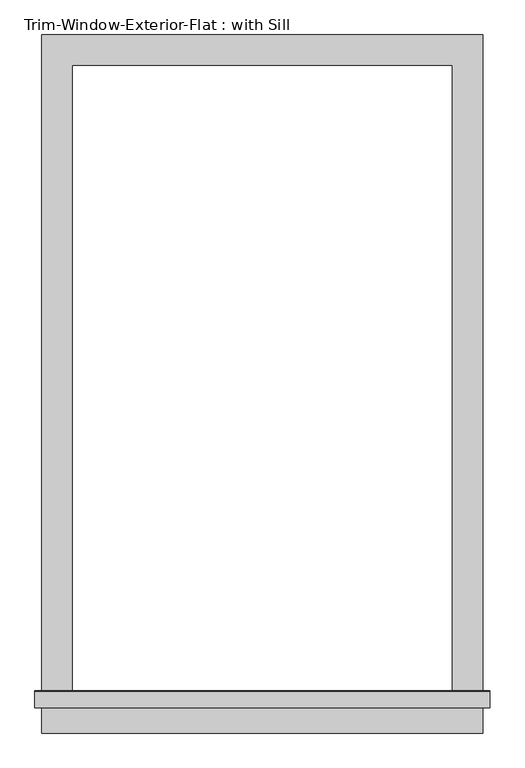
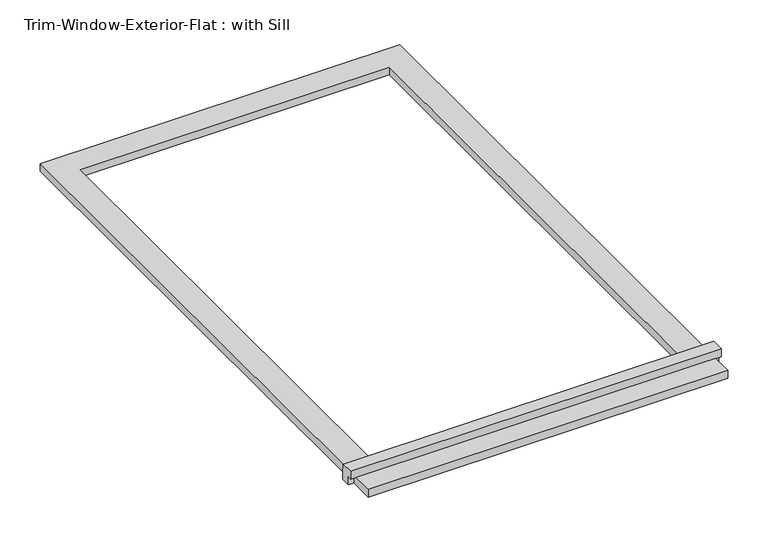
"""IFC4 building model written with IfcOpenShell, lengths in millimetres: proxy geometry, Trim-Window-Exterior-Flat : with Sill."""

from ifc_helpers import new_model, si_unit, frame, origin, origin_with_axes, place, context, project, spatial, polyline, outline, extrude, source, transform, mapped, element, save


def trim_window_exterior_flat_with_sill_68241f6a(model_context):
    return source(origin(), model_context, "Body", "SweptSolid", [
        extrude(outline(polyline([(412.75, -1190.5823709), (412.75, -1247.7323709), (-412.75, -1247.7323709), (-412.75, -1190.5823709), (412.75, -1190.5823709)])), origin_with_axes(), (0.0, 0.0, 1.0), 19.05),
        extrude(outline(polyline([(-1200.15, 38.1), (-1170.8580645, 38.1), (-1168.4, 19.05), (-1168.4, 0.0), (-1190.5823709, 0.0), (-1190.5823709, 19.05), (-1200.15, 19.05), (-1200.15, 38.1)])), frame((-425.45, 0.0, 0.0), z_axis=(1.0, 0.0, 0.0), x_axis=(0.0, 1.0, 0.0)), (0.0, 0.0, 1.0), 850.9),
        extrude(outline(polyline([(-412.75, 57.15), (412.75, 57.15), (412.75, -1168.4), (355.6, -1168.4), (355.6, 0.0), (-355.6, 0.0), (-355.6, -1168.4), (-412.75, -1168.4), (-412.75, 57.15)])), origin_with_axes(), (0.0, 0.0, 1.0), 19.05),
    ])


if __name__ == "__main__":
    model = new_model("IFC4")
    model_context = context("Model", 3, world=origin())
    ifc_project = project(units=[si_unit("LENGTHUNIT", "METRE", prefix="MILLI")], contexts=[model_context])
    site = spatial("IfcSite", under=ifc_project)
    building = spatial("IfcBuilding", under=site)
    placement = place(None, origin())
    trim_window_exterior_flat_with_sill_shape = trim_window_exterior_flat_with_sill_68241f6a(model_context)
    element("IfcBuildingElementProxy", 1, Name="Trim-Window-Exterior-Flat : with Sill", ObjectType="Trim-Window-Exterior-Flat : with Sill", at=placement, inside=building, context=model_context, shape_type="MappedRepresentation", body=[
        mapped(trim_window_exterior_flat_with_sill_shape, transform((0.0, 0.0, 0.0), x_axis=(1.0, 0.0, 0.0), y_axis=(0.0, 1.0, 0.0), z_axis=(0.0, 0.0, 1.0))),
    ])
    save(model, "model.ifc")

# Revit data of these elements
# Type "Trim-Window-Exterior-Flat : with Sill"
#   Trim Width = 0' - 2 1/4"
#   Trim Thickness_Picture Frame = 0' - 1 1/4"
#   Trim Thickness_with Sill = 0' - 0 3/4"
#   Sill Thickness = 0' - 1 1/4"
#   Opening Width [instance default] = 2' - 0"
#   Opening Height [instance default] = 3' - 0"
#   Default Elevation = 4' - 0"
#   Sill = yes
#   Picture Frame = no
#   Trim Material [instance default] = none
# Element 1 (IfcBuildingElementProxy, "Trim-Window-Exterior-Flat : with Sill")
#   Opening Width = 2' - 4"
#   Opening Height = 3' - 10"
#   Trim Material = Clad - White
#   Materials on its faces: "Clad - White"
# Materials
#   "Clad - White": class "Wood", colour RGB 242 242 238, transparency 0, Cost = 0
